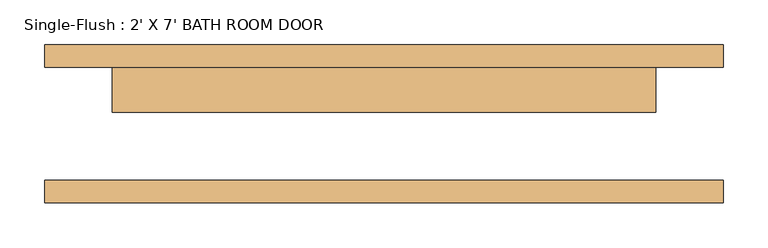
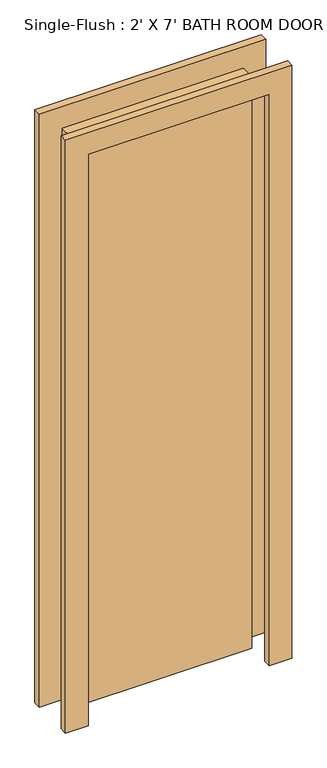
"""IFC4 building model written with IfcOpenShell, lengths in millimetres: door geometry, Single-Flush : 2' X 7' BATH ROOM DOOR."""

from ifc_helpers import new_model, si_unit, frame, origin, origin_with_axes, place, context, project, spatial, polyline, outline, extrude, source, transform, mapped, element, save


def single_flush_2_x_7_bath_room_door_025d1c86(model_context):
    return source(origin(), model_context, "Body", "SweptSolid", [
        extrude(outline(polyline([(2108.2, -381.0), (0.0, -381.0), (0.0, -304.8), (2032.0, -304.8), (2032.0, 304.8), (0.0, 304.8), (0.0, 381.0), (2108.2, 381.0), (2108.2, -381.0)])), frame((0.0, 63.5, 0.0), z_axis=(0.0, 1.0, 0.0), x_axis=(0.0, 0.0, 1.0)), (0.0, 0.0, 1.0), 25.4),
        extrude(outline(polyline([(2108.2, 381.0), (2108.2, -381.0), (0.0, -381.0), (0.0, -304.8), (2032.0, -304.8), (2032.0, 304.8), (0.0, 304.8), (0.0, 381.0), (2108.2, 381.0)])), frame((0.0, -88.9, 0.0), z_axis=(0.0, 1.0, 0.0), x_axis=(0.0, 0.0, 1.0)), (0.0, 0.0, 1.0), 25.4),
        extrude(outline(polyline([(304.8, 12.7), (-304.8, 12.7), (-304.8, 63.5), (304.8, 63.5), (304.8, 12.7)])), origin_with_axes(), (0.0, 0.0, 1.0), 2032.0),
    ])


if __name__ == "__main__":
    model = new_model("IFC4")
    model_context = context("Model", 3, world=origin())
    ifc_project = project(units=[si_unit("LENGTHUNIT", "METRE", prefix="MILLI")], contexts=[model_context])
    site = spatial("IfcSite", under=ifc_project)
    building = spatial("IfcBuilding", under=site)
    placement = place(None, origin())
    single_flush_2_x_7_bath_room_door_shape = single_flush_2_x_7_bath_room_door_025d1c86(model_context)
    element("IfcDoor", 1, ObjectType="Single-Flush : 2' X 7' BATH ROOM DOOR", at=placement, inside=building, context=model_context, shape_type="MappedRepresentation", body=[
        mapped(single_flush_2_x_7_bath_room_door_shape, transform((0.0, 0.0, 0.0), x_axis=(1.0, 0.0, 0.0), y_axis=(0.0, 1.0, 0.0), z_axis=(0.0, 0.0, 1.0))),
    ])
    save(model, "model.ifc")

# Revit data of these elements
# Type "Single-Flush : 2' X 7' BATH ROOM DOOR"
#   Type Mark = "11"
#   Construction Type Id = "MDOOR"
#   Assembly Code = "C1020"
#   Analytic Construction = "Metal"
#   Thickness = 0' - 2"
#   Heat Transfer Coefficient (U) = 0.651978 BTU/(h·ft²·°F)
#   Height = 6' - 8"
#   Trim Projection Ext = 0' - 1"
#   Trim Projection Int = 0' - 1"
#   Trim Width = 0' - 3"
#   Width = 2' - 0"
#   Define Thermal Properties by = 1
#   Door Material = Door - Panel
#   Frame Material = Door - Frame
#   Visual Light Transmittance = 0
#   Solar Heat Gain Coefficient = 0
#   Function = (empty or 0)
#   Wall Closure = (empty or 0)
# Element 1 (IfcDoor, "Single-Flush : 2' X 7' BATH ROOM DOOR")
#   Materials on its faces: "Door - Frame", "Door - Panel"
# Materials
#   "Door - Panel": class "Wood", colour RGB 210 159 95, transparency 0, Cost = 0
#   "Door - Frame": colour RGB 118 70 51, transparency 0, Cost = 0
